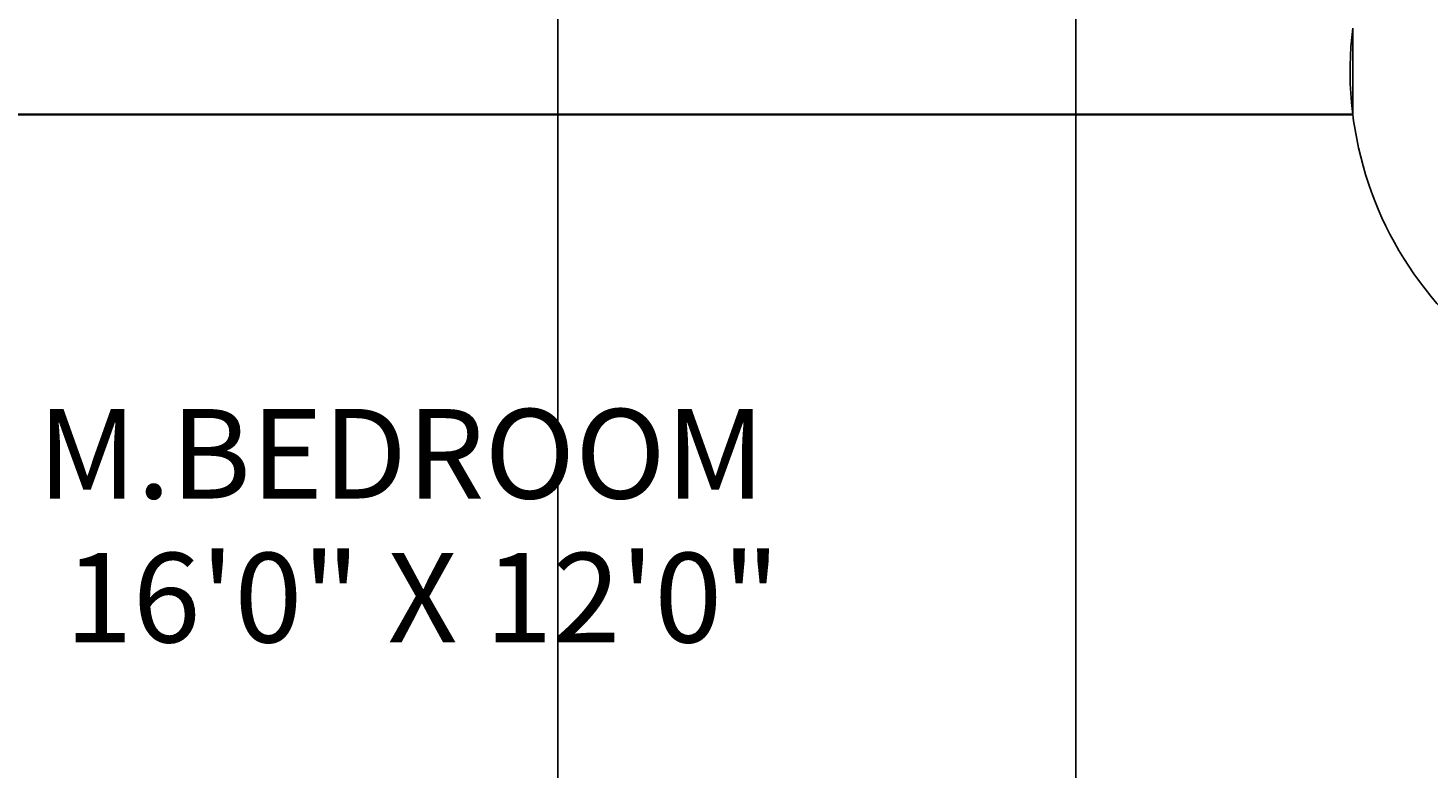
# Model space of a CAD drawing. Units: inches. Extents: x -61 to 1599, y -1316 to 257.
# Tile 55 of 204: x 143 to 240, y -334 to -282. Entities that reach past the tile are written whole.
import ezdxf

# ---------------------------------------------------------------- set-up
doc = ezdxf.new("R2010")
doc.units = ezdxf.units.IN
doc.header["$MEASUREMENT"] = 0
doc.linetypes.add('ACAD_ISO02W100', pattern=[15, 12, -3])
for name, color, linetype, lineweight in [('A-ANNO-DIMS', 2, 'Continuous', 18), ('A-AREA-IDEN', 1, 'Continuous', 18), ('A-WALL-JAMB', 4, 'ACAD_ISO02W100', 25), ('DOORS', 2, 'Continuous', 25), ('WALLS', 4, 'Continuous', 35)]:
    doc.layers.add(name, color=color, linetype=linetype, lineweight=lineweight)
doc.styles.get("Standard").update_dxf_attribs({"font": 'arial.ttf'})
doc.dimstyles.get("Standard").update_dxf_attribs({"dimtxt": 0.18, "dimasz": 0.18, "dimexe": 0.18, "dimexo": 0.0625, "dimgap": 0.09, "dimtad": 0, "dimtih": 1, "dimtoh": 1, "dimdec": 0, "dimzin": 0, "dimdsep": 46, "dimlunit": 3, "dimtxsty": 'Standard', "dimcen": 0.09, "dimadec": 0, "dimazin": 0, "dimtfac": 1, "dimtdec": 0, "dimtofl": 0, "dimtmove": 0, "dimatfit": 3, "dimfxl": 1, "dimtolj": 1, "dimtzin": 0, "dimarcsym": 0})

# ---------------------------------------------------------------- blocks, each defined once
blk = doc.blocks.new('DOOR-SWING-24')
blk.add_line((0, 0), (0, 3.6))
blk.add_lwpolyline([(0, 0), (0, -24), (1.05, -24), (1.05, 0)], close=True)
blk.add_arc((-0.441, 0.618), 24.622, 271.02591, 6.95592)
blk = doc.blocks.new('*D687')
at = {"layer": 'A-ANNO-DIMS', "color": 0, "lineweight": -2, "transparency": 16777216}
for p, q in [((289.418, 181.677), (-61.077, 181.677)), ((-60.897, 181.497), (-60.897, -528.952)), ((-60.897, -1239.765), (-60.897, -529.316)), ((319.64, -1239.945), (-61.077, -1239.945))]:
    blk.add_line(p, q, dxfattribs=at)
at = {"layer": 'A-ANNO-DIMS', "color": 0, "transparency": 16777216}
for points in [[(-60.927, 181.497), (-60.867, 181.497), (-60.897, 181.677)], [(-60.927, -1239.765), (-60.867, -1239.765), (-60.897, -1239.945)]]:
    blk.add_solid(points, dxfattribs=at)
at = {"layer": 'DEFPOINTS', "color": 0, "transparency": 16777216}
for p in [(289.481, 181.677), (-60.897, -1239.945), (319.703, -1239.945)]:
    blk.add_point(p, dxfattribs=at)
at = {"layer": 'A-ANNO-DIMS', "color": 0, "transparency": 16777216, "insert": (-60.897, -529.134), "char_height": 0.18, "attachment_point": 5}
blk.add_mtext('\\A1;1421.6', dxfattribs=at)
blk = doc.blocks.new('*D699')
at = {"layer": 'A-ANNO-DIMS', "color": 0, "lineweight": -2, "transparency": 16777216}
for p, q in [((835.64, -167.169), (-61.077, -167.169)), ((-60.897, -167.349), (-60.897, -306.726)), ((-60.897, -446.466), (-60.897, -307.09)), ((841.64, -446.646), (-61.077, -446.646))]:
    blk.add_line(p, q, dxfattribs=at)
at = {"layer": 'A-ANNO-DIMS', "color": 0, "transparency": 16777216}
for points in [[(-60.927, -167.349), (-60.867, -167.349), (-60.897, -167.169)], [(-60.927, -446.466), (-60.867, -446.466), (-60.897, -446.646)]]:
    blk.add_solid(points, dxfattribs=at)
at = {"layer": 'DEFPOINTS', "color": 0, "transparency": 16777216}
for p in [(835.703, -167.169), (-60.897, -446.646), (841.703, -446.646)]:
    blk.add_point(p, dxfattribs=at)
at = {"layer": 'A-ANNO-DIMS', "color": 0, "transparency": 16777216, "insert": (-60.897, -306.908), "char_height": 0.18, "attachment_point": 5}
blk.add_mtext('\\A1;279.5', dxfattribs=at)
blk = doc.blocks.new('*D700')
at = {"layer": 'A-ANNO-DIMS', "color": 0, "lineweight": -2, "transparency": 16777216}
for p, q in [((14.703, -616.882), (14.703, 257.457)), ((14.883, 257.277), (96.772, 257.277)), ((179.572, 257.277), (97.683, 257.277)), ((179.752, -616.882), (179.752, 257.457))]:
    blk.add_line(p, q, dxfattribs=at)
at = {"layer": 'A-ANNO-DIMS', "color": 0, "transparency": 16777216}
for points in [[(14.883, 257.307), (14.883, 257.247), (14.703, 257.277)], [(179.572, 257.307), (179.572, 257.247), (179.752, 257.277)]]:
    blk.add_solid(points, dxfattribs=at)
at = {"layer": 'DEFPOINTS', "color": 0, "transparency": 16777216}
for p in [(179.752, 257.277), (14.703, -616.945), (179.752, -616.945)]:
    blk.add_point(p, dxfattribs=at)
at = {"layer": 'A-ANNO-DIMS', "color": 0, "transparency": 16777216, "insert": (97.227, 257.277), "char_height": 0.18, "attachment_point": 5}
blk.add_mtext('\\A1;165.05', dxfattribs=at)
blk = doc.blocks.new('*D701')
at = {"layer": 'A-ANNO-DIMS', "color": 0, "lineweight": -2, "transparency": 16777216}
for p, q in [((215.752, -616.882), (215.752, 257.457)), ((215.932, 257.277), (233.924, 257.277)), ((252.702, 257.277), (234.711, 257.277)), ((252.882, -616.882), (252.882, 257.457))]:
    blk.add_line(p, q, dxfattribs=at)
at = {"layer": 'A-ANNO-DIMS', "color": 0, "transparency": 16777216}
for points in [[(215.932, 257.307), (215.932, 257.247), (215.752, 257.277)], [(252.702, 257.307), (252.702, 257.247), (252.882, 257.277)]]:
    blk.add_solid(points, dxfattribs=at)
at = {"layer": 'DEFPOINTS', "color": 0, "transparency": 16777216}
for p in [(252.882, 257.277), (215.752, -616.945), (252.882, -616.945)]:
    blk.add_point(p, dxfattribs=at)
at = {"layer": 'A-ANNO-DIMS', "color": 0, "transparency": 16777216, "insert": (234.317, 257.277), "char_height": 0.18, "attachment_point": 5}
blk.add_mtext('\\A1;37.13', dxfattribs=at)

msp = doc.modelspace()

# ---------------------------------------------------------------- linework, layer by layer
at = {"layer": 'A-WALL-JAMB'}
msp.add_line((234.999, -282.3229), (234.999, -288.3229), dxfattribs=at)
at = {"layer": 'WALLS'}
msp.add_line((87.7028, -288.3229), (235.0034, -288.3229), dxfattribs=at)

# ---------------------------------------------------------------- block references
at = {"layer": 'DOORS', "extrusion": (0, 0, -1), "zscale": -1}
msp.add_blockref('DOOR-SWING-24', (-258.999, -285.9229), dxfattribs=at)

# ---------------------------------------------------------------- texts
at = {"layer": 'A-AREA-IDEN'}
for s, height, p in [('M.BEDROOM ', 6.22364, (143.5758, -315.0227)), (' 16\'0" X 12\'0"', 6.223643, (143.5758, -325.0204))]:
    msp.add_text(s, height=height, dxfattribs=at).set_placement(p)

# ---------------------------------------------------------------- dimensions: what is measured, and where the dimension line sits
at = {"layer": 'A-ANNO-DIMS'}
for base, p1, p2, picture, middle in [((179.7521, 257.2771), (14.7028, -616.9446), (179.7521, -616.9446), '*D700', (97.2274, 257.2771)), ((252.8825, 257.2771), (215.7521, -616.9446), (252.8825, -616.9446), '*D701', (234.3173, 257.2771))]:
    dim = msp.add_linear_dim(base=base, p1=p1, p2=p2, dimstyle='Standard', override={"dimdec": 2, "dimlfac": 1, "dimrnd": 0, "dimzin": 0, "dimdsep": 46, "dimlunit": 2}, dxfattribs=at)
    dim.commit()
    dim.dimension.update_dxf_attribs({"geometry": picture, "text_midpoint": middle})
for base, p1, p2, picture, middle in [((-60.8972, -1239.9446), (289.4807, 181.6771), (319.7028, -1239.9446), '*D687', (-60.8972, -529.1337)), ((-60.8972, -446.6462), (835.7028, -167.169), (841.7028, -446.6462), '*D699', (-60.8972, -306.9076))]:
    dim = msp.add_linear_dim(base=base, p1=p1, p2=p2, angle=90, dimstyle='Standard', override={"dimdec": 1, "dimlfac": 1, "dimrnd": 0, "dimzin": 0, "dimdsep": 46, "dimlunit": 2}, dxfattribs=at)
    dim.commit()
    dim.dimension.update_dxf_attribs({"geometry": picture, "text_midpoint": middle})

doc.saveas('drawing.dxf')
